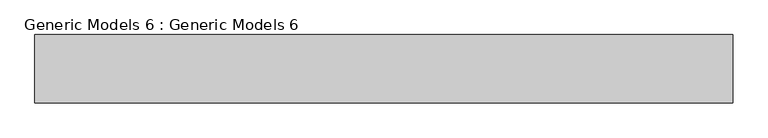
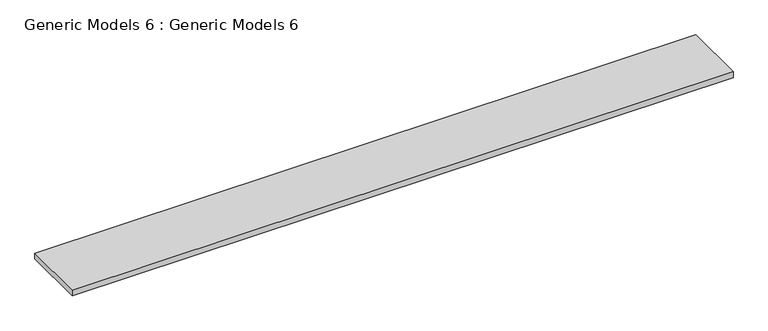
"""IFC4 building model written with IfcOpenShell, lengths in millimetres: proxy geometry, Generic Models 6 : Generic Models 6."""

from ifc_helpers import new_model, si_unit, frame, origin, place, context, project, spatial, polyline, outline, extrude, source, transform, mapped, element, save


def generic_models_6_generic_models_6_790b48f3(model_context):
    return source(origin(), model_context, "Body", "SweptSolid", [
        extrude(outline(polyline([(-8791.3780416, -14017.5239804), (-8791.3780416, -12374.29161), (8031.1066869, -12374.29161), (8031.1066869, -14017.5239804), (-8791.3780416, -14017.5239804)])), frame((0.0, 0.0, -152.4), z_axis=(0.0, 0.0, 1.0), x_axis=(1.0, 0.0, 0.0)), (0.0, 0.0, 1.0), 152.4),
    ])


if __name__ == "__main__":
    model = new_model("IFC4")
    model_context = context("Model", 3, world=origin())
    ifc_project = project(units=[si_unit("LENGTHUNIT", "METRE", prefix="MILLI")], contexts=[model_context])
    site = spatial("IfcSite", under=ifc_project)
    building = spatial("IfcBuilding", under=site)
    placement = place(None, origin())
    generic_models_6_generic_models_6_shape = generic_models_6_generic_models_6_790b48f3(model_context)
    element("IfcBuildingElementProxy", 1, Name="Generic Models 6 : Generic Models 6", ObjectType="Generic Models 6 : Generic Models 6", at=placement, inside=building, context=model_context, shape_type="MappedRepresentation", body=[
        mapped(generic_models_6_generic_models_6_shape, transform((0.0, 0.0, 0.0), x_axis=(1.0, 0.0, 0.0), y_axis=(0.0, 1.0, 0.0), z_axis=(0.0, 0.0, 1.0))),
    ])
    save(model, "model.ifc")
